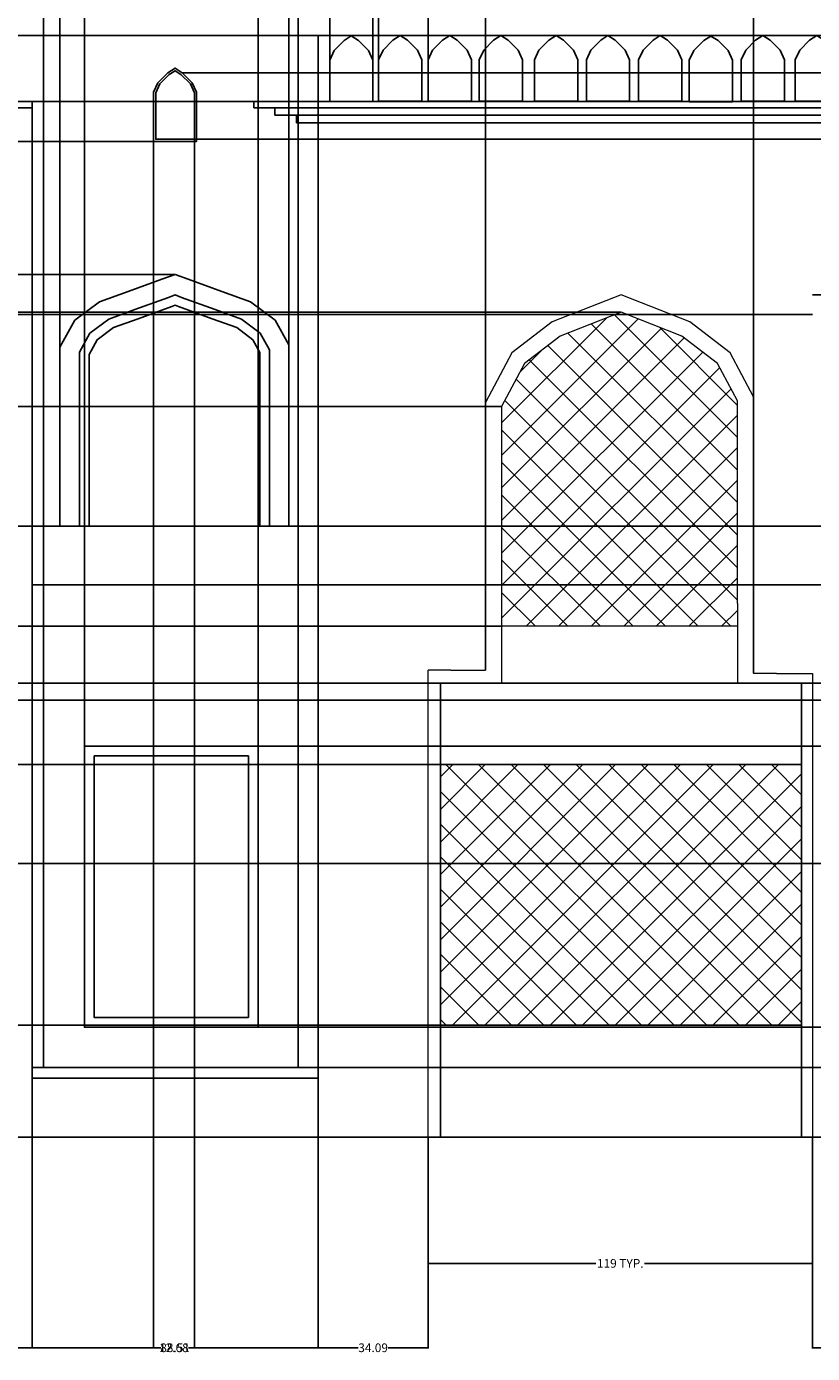
# Model space of a CAD drawing. Units: inches. Extents: x 2 to 1442, y 20 to 729.
# Tile 3 of 8: x 343 to 586, y 20 to 431. Entities that reach past the tile are written whole.
import ezdxf

# ---------------------------------------------------------------- set-up
doc = ezdxf.new("R2010")
doc.units = ezdxf.units.IN
doc.header["$MEASUREMENT"] = 0
for name, color, linetype, lineweight in [('A-ANNO-DIMS', 2, 'Continuous', 18), ('A-ELEV', 7, 'Continuous', 25), ('A-GLAZ', 4, 'Continuous', 18), ('A-GLAZ-PATT', 9, 'Continuous', 13)]:
    doc.layers.add(name, color=color, linetype=linetype, lineweight=lineweight)
doc.styles.get("Standard").update_dxf_attribs({"font": 'arial.ttf'})
doc.dimstyles.get("Standard").update_dxf_attribs({"dimtxt": 2.6875, "dimasz": 0.18, "dimexe": 0.18, "dimexo": 0.0625, "dimgap": 0.09, "dimtad": 0, "dimtih": 1, "dimtoh": 1, "dimdec": 4, "dimzin": 0, "dimdsep": 46, "dimlunit": 4, "dimtxsty": 'Standard', "dimcen": 0.09, "dimadec": 0, "dimazin": 0, "dimtfac": 1, "dimtdec": 4, "dimtofl": 0, "dimtmove": 0, "dimatfit": 3, "dimfxl": 1, "dimtolj": 1, "dimtzin": 0, "dimarcsym": 0})

# ---------------------------------------------------------------- blocks, each defined once
blk = doc.blocks.new('WIN-JALI-PANEL')
for p, q in [((17.71, 144.52), (17.71, 165.38)), ((22.71, 165.38), (22.71, 158.15)), ((95.66, 165.25), (95.66, 158.15)), ((100.66, 165.25), (100.66, 143.52)), ((95.66, 158.15), (22.71, 158.15)), ((22.71, 158.15), (22.71, 140.52)), ((95.66, 158.15), (95.66, 140.52)), ((0, 0), (0, 144.52)), ((7.01, 144.52), (0, 144.52)), ((7.01, 144.52), (17.71, 144.52)), ((107.81, 143.52), (100.66, 143.52)), ((107.81, 143.52), (118.87, 143.52)), ((118.87, 143.52), (118.87, 100.88)), ((118.87, 100.88), (118.87, 0))]:
    blk.add_line(p, q)
for points in [[(100.66, 165.25), (100.66, 224.45), (100.65, 229.2), (93.44, 242.86), (80.93, 252.42), (59.66, 260.79), (38.39, 252.42), (25.88, 242.86), (17.71, 227.39), (17.71, 165.38)], [(95.66, 165.25), (95.66, 224.45), (95.66, 227.96), (89.53, 239.55), (78.45, 248.02), (59.66, 255.41), (40.87, 248.02), (29.79, 239.55), (22.71, 226.15), (22.71, 165.38)]]:
    blk.add_lwpolyline(points)
blk = doc.blocks.new('*D9')
at = {"layer": 'A-ANNO-DIMS', "color": 0, "lineweight": -2, "transparency": 16777216}
for p, q in [((585.99, 348.06), (625.22, 348.06)), ((625.04, 347.88), (625.04, 219.14)), ((625.04, 87.45), (625.04, 216.18)), ((585.99, 87.27), (625.22, 87.27))]:
    blk.add_line(p, q, dxfattribs=at)
at = {"layer": 'A-ANNO-DIMS', "color": 0, "transparency": 16777216}
for points in [[(625.01, 347.88), (625.07, 347.88), (625.04, 348.06)], [(625.01, 87.45), (625.07, 87.45), (625.04, 87.27)]]:
    blk.add_solid(points, dxfattribs=at)
at = {"layer": 'Defpoints', "color": 0, "transparency": 16777216}
for p in [(585.93, 348.06), (625.04, 348.06), (585.93, 87.27)]:
    blk.add_point(p, dxfattribs=at)
at = {"layer": 'A-ANNO-DIMS', "color": 0, "transparency": 16777216, "insert": (625.04, 217.66), "char_height": 2.6875, "attachment_point": 5}
blk.add_mtext('\\A1;JALI SCREEN 261 TYP.', dxfattribs=at)
blk = doc.blocks.new('*D10')
at = {"layer": 'A-ANNO-DIMS', "color": 0, "lineweight": -2, "transparency": 16777216}
for p, q in [((467.06, 87.21), (467.06, 47.97)), ((585.93, 87.21), (585.93, 47.97)), ((467.24, 48.15), (518.94, 48.15)), ((585.75, 48.15), (534.04, 48.15))]:
    blk.add_line(p, q, dxfattribs=at)
at = {"layer": 'A-ANNO-DIMS', "color": 0, "transparency": 16777216}
for points in [[(467.24, 48.18), (467.24, 48.12), (467.06, 48.15)], [(585.75, 48.18), (585.75, 48.12), (585.93, 48.15)]]:
    blk.add_solid(points, dxfattribs=at)
at = {"layer": 'Defpoints', "color": 0, "transparency": 16777216}
for p in [(467.06, 87.27), (585.93, 87.27), (585.93, 48.15)]:
    blk.add_point(p, dxfattribs=at)
at = {"layer": 'A-ANNO-DIMS', "color": 0, "transparency": 16777216, "insert": (526.49, 48.15), "char_height": 2.6875, "attachment_point": 5}
blk.add_mtext('\\A1;119 TYP.', dxfattribs=at)
blk = doc.blocks.new('*D18')
at = {"layer": 'A-ANNO-DIMS', "color": 0, "lineweight": -2, "transparency": 16777216}
for p, q in [((318.25, 87.21), (318.25, 21.84)), ((344.45, 87.21), (344.45, 21.84)), ((318.43, 22.02), (325.66, 22.02)), ((344.27, 22.02), (337.04, 22.02))]:
    blk.add_line(p, q, dxfattribs=at)
at = {"layer": 'A-ANNO-DIMS', "color": 0, "transparency": 16777216}
for points in [[(318.43, 22.05), (318.43, 21.99), (318.25, 22.02)], [(344.27, 22.05), (344.27, 21.99), (344.45, 22.02)]]:
    blk.add_solid(points, dxfattribs=at)
at = {"layer": 'Defpoints', "color": 0, "transparency": 16777216}
for p in [(318.25, 87.27), (344.45, 87.27), (344.45, 22.02)]:
    blk.add_point(p, dxfattribs=at)
at = {"layer": 'A-ANNO-DIMS', "color": 0, "transparency": 16777216, "insert": (331.35, 22.02), "char_height": 2.688, "attachment_point": 5}
blk.add_mtext('\\A1;26.204', dxfattribs=at)
blk = doc.blocks.new('*D19')
at = {"layer": 'A-ANNO-DIMS', "color": 0, "lineweight": -2, "transparency": 16777216}
for p, q in [((344.45, 87.21), (344.45, 21.84)), ((432.97, 87.21), (432.97, 21.84)), ((344.63, 22.02), (384.34, 22.02)), ((432.79, 22.02), (393.08, 22.02))]:
    blk.add_line(p, q, dxfattribs=at)
at = {"layer": 'A-ANNO-DIMS', "color": 0, "transparency": 16777216}
for points in [[(344.63, 22.05), (344.63, 21.99), (344.45, 22.02)], [(432.79, 22.05), (432.79, 21.99), (432.97, 22.02)]]:
    blk.add_solid(points, dxfattribs=at)
at = {"layer": 'Defpoints', "color": 0, "transparency": 16777216}
for p in [(344.45, 87.27), (432.97, 87.27), (432.97, 22.02)]:
    blk.add_point(p, dxfattribs=at)
at = {"layer": 'A-ANNO-DIMS', "color": 0, "transparency": 16777216, "insert": (388.71, 22.02), "char_height": 2.688, "attachment_point": 5}
blk.add_mtext('\\A1;88.51', dxfattribs=at)
blk = doc.blocks.new('*D20')
at = {"layer": 'A-ANNO-DIMS', "color": 0, "lineweight": -2, "transparency": 16777216}
for p, q in [((432.97, 87.21), (432.97, 21.84)), ((467.06, 87.21), (467.06, 21.84)), ((433.15, 22.02), (445.39, 22.02)), ((466.88, 22.02), (454.64, 22.02))]:
    blk.add_line(p, q, dxfattribs=at)
at = {"layer": 'A-ANNO-DIMS', "color": 0, "transparency": 16777216}
for points in [[(433.15, 22.05), (433.15, 21.99), (432.97, 22.02)], [(466.88, 22.05), (466.88, 21.99), (467.06, 22.02)]]:
    blk.add_solid(points, dxfattribs=at)
at = {"layer": 'Defpoints', "color": 0, "transparency": 16777216}
for p in [(432.97, 87.27), (467.06, 87.27), (467.06, 22.02)]:
    blk.add_point(p, dxfattribs=at)
at = {"layer": 'A-ANNO-DIMS', "color": 0, "transparency": 16777216, "insert": (450.01, 22.02), "char_height": 2.688, "attachment_point": 5}
blk.add_mtext('\\A1;34.09', dxfattribs=at)
blk = doc.blocks.new('*D21')
at = {"layer": 'A-ANNO-DIMS', "color": 0, "lineweight": -2, "transparency": 16777216}
for p, q in [((585.93, 87.21), (585.93, 21.84)), ((656, 87.21), (656, 21.84)), ((586.11, 22.02), (616.35, 22.02)), ((655.82, 22.02), (625.58, 22.02))]:
    blk.add_line(p, q, dxfattribs=at)
at = {"layer": 'A-ANNO-DIMS', "color": 0, "transparency": 16777216}
for points in [[(586.11, 22.05), (586.11, 21.99), (585.93, 22.02)], [(655.82, 22.05), (655.82, 21.99), (656, 22.02)]]:
    blk.add_solid(points, dxfattribs=at)
at = {"layer": 'Defpoints', "color": 0, "transparency": 16777216}
for p in [(585.93, 87.27), (656, 87.27), (656, 22.02)]:
    blk.add_point(p, dxfattribs=at)
at = {"layer": 'A-ANNO-DIMS', "color": 0, "transparency": 16777216, "insert": (620.96, 22.02), "char_height": 2.688, "attachment_point": 5}
blk.add_mtext('\\A1;70.07', dxfattribs=at)
blk = doc.blocks.new('*D49')
at = {"layer": 'A-ANNO-DIMS', "color": 0, "lineweight": -2, "transparency": 16777216}
for p, q in [((353.09, 276.51), (353.09, 726.93)), ((353.27, 726.75), (383.9, 726.75)), ((423.76, 726.75), (393.14, 726.75)), ((423.94, 276.51), (423.94, 726.93))]:
    blk.add_line(p, q, dxfattribs=at)
at = {"layer": 'A-ANNO-DIMS', "color": 0, "transparency": 16777216}
for points in [[(353.27, 726.78), (353.27, 726.72), (353.09, 726.75)], [(423.76, 726.78), (423.76, 726.72), (423.94, 726.75)]]:
    blk.add_solid(points, dxfattribs=at)
at = {"layer": 'Defpoints', "color": 0, "transparency": 16777216}
for p in [(423.94, 726.75), (353.09, 276.44), (423.94, 276.44)]:
    blk.add_point(p, dxfattribs=at)
at = {"layer": 'A-ANNO-DIMS', "color": 0, "transparency": 16777216, "insert": (388.52, 726.75), "char_height": 2.688, "attachment_point": 5}
blk.add_mtext('\\A1;70.85', dxfattribs=at)
blk = doc.blocks.new('*D50')
at = {"layer": 'A-ANNO-DIMS', "color": 0, "lineweight": -2, "transparency": 16777216}
for p, q in [((433.03, 108.8), (1436.55, 108.8)), ((1436.37, 108.62), (1436.37, 99.5)), ((1436.37, 87.45), (1436.37, 96.57)), ((433.03, 87.27), (1436.55, 87.27))]:
    blk.add_line(p, q, dxfattribs=at)
at = {"layer": 'A-ANNO-DIMS', "color": 0, "transparency": 16777216}
for points in [[(1436.34, 108.62), (1436.4, 108.62), (1436.37, 108.8)], [(1436.34, 87.45), (1436.4, 87.45), (1436.37, 87.27)]]:
    blk.add_solid(points, dxfattribs=at)
at = {"layer": 'Defpoints', "color": 0, "transparency": 16777216}
for p in [(432.97, 108.8), (1436.37, 108.8), (432.97, 87.27)]:
    blk.add_point(p, dxfattribs=at)
at = {"layer": 'A-ANNO-DIMS', "color": 0, "transparency": 16777216, "insert": (1436.37, 98.04), "char_height": 2.688, "attachment_point": 5}
blk.add_mtext('\\A1;21.53', dxfattribs=at)
blk = doc.blocks.new('*D51')
at = {"layer": 'A-ANNO-DIMS', "color": 0, "lineweight": -2, "transparency": 16777216}
for p, q in [((426.83, 227.79), (1436.55, 227.79)), ((1436.37, 227.61), (1436.37, 169.76)), ((1436.37, 108.98), (1436.37, 166.83)), ((433.03, 108.8), (1436.55, 108.8))]:
    blk.add_line(p, q, dxfattribs=at)
at = {"layer": 'A-ANNO-DIMS', "color": 0, "transparency": 16777216}
for points in [[(1436.34, 227.61), (1436.4, 227.61), (1436.37, 227.79)], [(1436.34, 108.98), (1436.4, 108.98), (1436.37, 108.8)]]:
    blk.add_solid(points, dxfattribs=at)
at = {"layer": 'Defpoints', "color": 0, "transparency": 16777216}
for p in [(426.77, 227.79), (1436.37, 227.79), (432.97, 108.8)]:
    blk.add_point(p, dxfattribs=at)
at = {"layer": 'A-ANNO-DIMS', "color": 0, "transparency": 16777216, "insert": (1436.37, 168.3), "char_height": 2.688, "attachment_point": 5}
blk.add_mtext('\\A1;118.99', dxfattribs=at)
blk = doc.blocks.new('*D52')
at = {"layer": 'A-ANNO-DIMS', "color": 0, "lineweight": -2, "transparency": 16777216}
for p, q in [((433.03, 258.25), (1436.55, 258.25)), ((1436.37, 258.07), (1436.37, 244.49)), ((1436.37, 227.97), (1436.37, 241.56)), ((426.83, 227.79), (1436.55, 227.79))]:
    blk.add_line(p, q, dxfattribs=at)
at = {"layer": 'A-ANNO-DIMS', "color": 0, "transparency": 16777216}
for points in [[(1436.34, 258.07), (1436.4, 258.07), (1436.37, 258.25)], [(1436.34, 227.97), (1436.4, 227.97), (1436.37, 227.79)]]:
    blk.add_solid(points, dxfattribs=at)
at = {"layer": 'Defpoints', "color": 0, "transparency": 16777216}
for p in [(432.97, 258.25), (1436.37, 258.25), (426.77, 227.79)]:
    blk.add_point(p, dxfattribs=at)
at = {"layer": 'A-ANNO-DIMS', "color": 0, "transparency": 16777216, "insert": (1436.37, 243.02), "char_height": 2.688, "attachment_point": 5}
blk.add_mtext('\\A1;30.464', dxfattribs=at)
blk = doc.blocks.new('*D53')
at = {"layer": 'A-ANNO-DIMS', "color": 0, "lineweight": -2, "transparency": 16777216}
for p, q in [((433.03, 276.44), (1436.55, 276.44)), ((1436.37, 276.26), (1436.37, 268.81)), ((1436.37, 258.43), (1436.37, 265.89)), ((433.03, 258.25), (1436.55, 258.25))]:
    blk.add_line(p, q, dxfattribs=at)
at = {"layer": 'A-ANNO-DIMS', "color": 0, "transparency": 16777216}
for points in [[(1436.34, 276.26), (1436.4, 276.26), (1436.37, 276.44)], [(1436.34, 258.43), (1436.4, 258.43), (1436.37, 258.25)]]:
    blk.add_solid(points, dxfattribs=at)
at = {"layer": 'Defpoints', "color": 0, "transparency": 16777216}
for p in [(432.97, 276.44), (1436.37, 276.44), (432.97, 258.25)]:
    blk.add_point(p, dxfattribs=at)
at = {"layer": 'A-ANNO-DIMS', "color": 0, "transparency": 16777216, "insert": (1436.37, 267.35), "char_height": 2.688, "attachment_point": 5}
blk.add_mtext('\\A1;18.19', dxfattribs=at)
blk = doc.blocks.new('*D54')
at = {"layer": 'A-ANNO-DIMS', "color": 0, "lineweight": -2, "transparency": 16777216}
for p, q in [((388.65, 354.39), (7.1, 354.39)), ((7.28, 354.21), (7.28, 316.88)), ((7.28, 276.62), (7.28, 313.95)), ((353.03, 276.44), (7.1, 276.44))]:
    blk.add_line(p, q, dxfattribs=at)
at = {"layer": 'A-ANNO-DIMS', "color": 0, "transparency": 16777216}
for points in [[(7.25, 354.21), (7.31, 354.21), (7.28, 354.39)], [(7.25, 276.62), (7.31, 276.62), (7.28, 276.44)]]:
    blk.add_solid(points, dxfattribs=at)
at = {"layer": 'Defpoints', "color": 0, "transparency": 16777216}
for p in [(7.28, 354.39), (388.71, 354.39), (353.09, 276.44)]:
    blk.add_point(p, dxfattribs=at)
at = {"layer": 'A-ANNO-DIMS', "color": 0, "transparency": 16777216, "insert": (7.28, 315.41), "char_height": 2.688, "attachment_point": 5}
blk.add_mtext('\\A1;77.94', dxfattribs=at)
blk = doc.blocks.new('*D55')
at = {"layer": 'A-ANNO-DIMS', "color": 0, "lineweight": -2, "transparency": 16777216}
for p, q in [((391.01, 416.82), (1436.55, 416.82)), ((1436.37, 416.64), (1436.37, 407.98)), ((1436.37, 396.4), (1436.37, 405.06)), ((394.77, 396.22), (1436.55, 396.22))]:
    blk.add_line(p, q, dxfattribs=at)
at = {"layer": 'A-ANNO-DIMS', "color": 0, "transparency": 16777216}
for points in [[(1436.34, 416.64), (1436.4, 416.64), (1436.37, 416.82)], [(1436.34, 396.4), (1436.4, 396.4), (1436.37, 396.22)]]:
    blk.add_solid(points, dxfattribs=at)
at = {"layer": 'Defpoints', "color": 0, "transparency": 16777216}
for p in [(390.95, 416.82), (1436.37, 416.82), (394.7, 396.22)]:
    blk.add_point(p, dxfattribs=at)
at = {"layer": 'A-ANNO-DIMS', "color": 0, "transparency": 16777216, "insert": (1436.37, 406.52), "char_height": 2.688, "attachment_point": 5}
blk.add_mtext('\\A1;20.605', dxfattribs=at)
blk = doc.blocks.new('*D56')
at = {"layer": 'A-ANNO-DIMS', "color": 0, "lineweight": -2, "transparency": 16777216}
for p, q in [((382.02, 395.46), (382.02, 21.84)), ((394.7, 396.15), (394.7, 21.84)), ((382.2, 22.02), (383.86, 22.02)), ((394.52, 22.02), (392.86, 22.02))]:
    blk.add_line(p, q, dxfattribs=at)
at = {"layer": 'A-ANNO-DIMS', "color": 0, "transparency": 16777216}
for points in [[(382.2, 22.05), (382.2, 21.99), (382.02, 22.02)], [(394.52, 22.05), (394.52, 21.99), (394.7, 22.02)]]:
    blk.add_solid(points, dxfattribs=at)
at = {"layer": 'Defpoints', "color": 0, "transparency": 16777216}
for p in [(382.02, 395.53), (394.7, 396.22), (394.7, 22.02)]:
    blk.add_point(p, dxfattribs=at)
at = {"layer": 'A-ANNO-DIMS', "color": 0, "transparency": 16777216, "insert": (388.36, 22.02), "char_height": 2.688, "attachment_point": 5}
blk.add_mtext('\\A1;12.68', dxfattribs=at)
blk = doc.blocks.new('*D57')
at = {"layer": 'A-ANNO-DIMS', "color": 0, "lineweight": -2, "transparency": 16777216}
for p, q in [((381.96, 395.53), (7.1, 395.53)), ((7.28, 395.35), (7.28, 376.4)), ((7.28, 354.57), (7.28, 373.52)), ((388.65, 354.39), (7.1, 354.39))]:
    blk.add_line(p, q, dxfattribs=at)
at = {"layer": 'A-ANNO-DIMS', "color": 0, "transparency": 16777216}
for points in [[(7.25, 395.35), (7.31, 395.35), (7.28, 395.53)], [(7.25, 354.57), (7.31, 354.57), (7.28, 354.39)]]:
    blk.add_solid(points, dxfattribs=at)
at = {"layer": 'Defpoints', "color": 0, "transparency": 16777216}
for p in [(382.02, 395.53), (7.28, 354.39), (388.71, 354.39)]:
    blk.add_point(p, dxfattribs=at)
at = {"layer": 'A-ANNO-DIMS', "color": 0, "transparency": 16777216, "insert": (7.28, 374.96), "char_height": 2.688, "attachment_point": 5}
blk.add_mtext('\\A1;41.14', dxfattribs=at)
blk = doc.blocks.new('*D58')
at = {"layer": 'A-ANNO-DIMS', "color": 0, "lineweight": -2, "transparency": 16777216}
for p, q in [((347.98, 227.85), (347.98, 726.93)), ((348.16, 726.75), (382.76, 726.75)), ((426.59, 726.75), (391.99, 726.75)), ((426.77, 227.85), (426.77, 726.93))]:
    blk.add_line(p, q, dxfattribs=at)
at = {"layer": 'A-ANNO-DIMS', "color": 0, "transparency": 16777216}
for points in [[(348.16, 726.78), (348.16, 726.72), (347.98, 726.75)], [(426.59, 726.78), (426.59, 726.72), (426.77, 726.75)]]:
    blk.add_solid(points, dxfattribs=at)
at = {"layer": 'Defpoints', "color": 0, "transparency": 16777216}
for p in [(426.77, 726.75), (347.98, 227.79), (426.77, 227.79)]:
    blk.add_point(p, dxfattribs=at)
at = {"layer": 'A-ANNO-DIMS', "color": 0, "transparency": 16777216, "insert": (387.38, 726.75), "char_height": 2.688, "attachment_point": 5}
blk.add_mtext('\\A1;78.79', dxfattribs=at)
blk = doc.blocks.new('*D59')
at = {"layer": 'A-ANNO-DIMS', "color": 0, "lineweight": -2, "transparency": 16777216}
for p, q in [((360.68, 208.33), (360.68, 726.93)), ((360.86, 726.75), (382.91, 726.75)), ((414.24, 726.75), (392.18, 726.75)), ((414.42, 208.33), (414.42, 726.93))]:
    blk.add_line(p, q, dxfattribs=at)
at = {"layer": 'A-ANNO-DIMS', "color": 0, "transparency": 16777216}
for points in [[(360.86, 726.78), (360.86, 726.72), (360.68, 726.75)], [(414.24, 726.78), (414.24, 726.72), (414.42, 726.75)]]:
    blk.add_solid(points, dxfattribs=at)
at = {"layer": 'Defpoints', "color": 0, "transparency": 16777216}
for p in [(414.42, 726.75), (360.68, 208.27), (414.42, 208.27)]:
    blk.add_point(p, dxfattribs=at)
at = {"layer": 'A-ANNO-DIMS', "color": 0, "transparency": 16777216, "insert": (387.55, 726.75), "char_height": 2.688, "attachment_point": 5}
blk.add_mtext('\\A1;53.75', dxfattribs=at)
blk = doc.blocks.new('*D60')
at = {"layer": 'A-ANNO-DIMS', "color": 0, "lineweight": -2, "transparency": 16777216}
for p, q in [((414.48, 208.27), (1436.55, 208.27)), ((1436.37, 208.09), (1436.37, 166.24)), ((1436.37, 121.46), (1436.37, 163.32)), ((414.48, 121.28), (1436.55, 121.28))]:
    blk.add_line(p, q, dxfattribs=at)
at = {"layer": 'A-ANNO-DIMS', "color": 0, "transparency": 16777216}
for points in [[(1436.34, 208.09), (1436.4, 208.09), (1436.37, 208.27)], [(1436.34, 121.46), (1436.4, 121.46), (1436.37, 121.28)]]:
    blk.add_solid(points, dxfattribs=at)
at = {"layer": 'Defpoints', "color": 0, "transparency": 16777216}
for p in [(414.42, 208.27), (1436.37, 208.27), (414.42, 121.28)]:
    blk.add_point(p, dxfattribs=at)
at = {"layer": 'A-ANNO-DIMS', "color": 0, "transparency": 16777216, "insert": (1436.37, 164.78), "char_height": 2.688, "attachment_point": 5}
blk.add_mtext('\\A1;86.99', dxfattribs=at)
blk = doc.blocks.new('*D61')
at = {"layer": 'A-ANNO-DIMS', "color": 0, "lineweight": -2, "transparency": 16777216}
for p, q in [((432.9, 428.31), (7.1, 428.31)), ((7.28, 428.13), (7.28, 419.56)), ((7.28, 408.07), (7.28, 416.64)), ((432.9, 407.89), (7.1, 407.89))]:
    blk.add_line(p, q, dxfattribs=at)
at = {"layer": 'A-ANNO-DIMS', "color": 0, "transparency": 16777216}
for points in [[(7.25, 428.13), (7.31, 428.13), (7.28, 428.31)], [(7.25, 408.07), (7.31, 408.07), (7.28, 407.89)]]:
    blk.add_solid(points, dxfattribs=at)
at = {"layer": 'Defpoints', "color": 0, "transparency": 16777216}
for p in [(7.28, 428.31), (432.97, 428.31), (432.97, 407.89)]:
    blk.add_point(p, dxfattribs=at)
at = {"layer": 'A-ANNO-DIMS', "color": 0, "transparency": 16777216, "insert": (7.28, 418.1), "char_height": 2.688, "attachment_point": 5}
blk.add_mtext('\\A1;20.426', dxfattribs=at)
blk = doc.blocks.new('*D62')
at = {"layer": 'A-ANNO-DIMS', "color": 0, "lineweight": -2, "transparency": 16777216}
for p, q in [((436.57, 420.81), (436.57, 726.93)), ((436.75, 726.75), (438.76, 726.75)), ((449.76, 726.75), (447.75, 726.75)), ((449.94, 420.81), (449.94, 726.93))]:
    blk.add_line(p, q, dxfattribs=at)
at = {"layer": 'A-ANNO-DIMS', "color": 0, "transparency": 16777216}
for points in [[(436.75, 726.78), (436.75, 726.72), (436.57, 726.75)], [(449.76, 726.78), (449.76, 726.72), (449.94, 726.75)]]:
    blk.add_solid(points, dxfattribs=at)
at = {"layer": 'Defpoints', "color": 0, "transparency": 16777216}
for p in [(449.94, 726.75), (436.57, 420.75), (449.94, 420.75)]:
    blk.add_point(p, dxfattribs=at)
at = {"layer": 'A-ANNO-DIMS', "color": 0, "transparency": 16777216, "insert": (443.26, 726.75), "char_height": 2.688, "attachment_point": 5}
blk.add_mtext('\\A1;13.37', dxfattribs=at)
blk = doc.blocks.new('*D63')
at = {"layer": 'A-ANNO-DIMS', "color": 0, "lineweight": -2, "transparency": 16777216}
for p, q in [((451.71, 420.89), (451.71, 726.93)), ((451.89, 726.75), (454.89, 726.75)), ((466.88, 726.75), (463.88, 726.75)), ((467.06, 420.89), (467.06, 726.93))]:
    blk.add_line(p, q, dxfattribs=at)
at = {"layer": 'A-ANNO-DIMS', "color": 0, "transparency": 16777216}
for points in [[(451.89, 726.78), (451.89, 726.72), (451.71, 726.75)], [(466.88, 726.78), (466.88, 726.72), (467.06, 726.75)]]:
    blk.add_solid(points, dxfattribs=at)
at = {"layer": 'Defpoints', "color": 0, "transparency": 16777216}
for p in [(467.06, 726.75), (451.71, 420.83), (467.06, 420.83)]:
    blk.add_point(p, dxfattribs=at)
at = {"layer": 'A-ANNO-DIMS', "color": 0, "transparency": 16777216, "insert": (459.39, 726.75), "char_height": 2.688, "attachment_point": 5}
blk.add_mtext('\\A1;15.34', dxfattribs=at)
blk = doc.blocks.new('*D72')
at = {"layer": 'A-ANNO-DIMS', "color": 0, "lineweight": -2, "transparency": 16777216}
for p, q in [((585.94, 341.99), (7.1, 341.99)), ((7.28, 341.81), (7.28, 216.09)), ((7.28, 87.45), (7.28, 213.17)), ((592.44, 87.27), (7.1, 87.27))]:
    blk.add_line(p, q, dxfattribs=at)
at = {"layer": 'A-ANNO-DIMS', "color": 0, "transparency": 16777216}
for points in [[(7.25, 341.81), (7.31, 341.81), (7.28, 341.99)], [(7.25, 87.45), (7.31, 87.45), (7.28, 87.27)]]:
    blk.add_solid(points, dxfattribs=at)
at = {"layer": 'Defpoints', "color": 0, "transparency": 16777216}
for p in [(7.28, 341.99), (586, 341.99), (592.5, 87.27)]:
    blk.add_point(p, dxfattribs=at)
at = {"layer": 'A-ANNO-DIMS', "color": 0, "transparency": 16777216, "insert": (7.28, 214.63), "char_height": 2.688, "attachment_point": 5}
blk.add_mtext('\\A1;254.7', dxfattribs=at)
blk = doc.blocks.new('*D74')
at = {"layer": 'A-ANNO-DIMS', "color": 0, "lineweight": -2, "transparency": 16777216}
for p, q in [((655.94, 172), (7.1, 172)), ((7.28, 171.82), (7.28, 131.1)), ((7.28, 87.45), (7.28, 128.17)), ((655.94, 87.27), (7.1, 87.27))]:
    blk.add_line(p, q, dxfattribs=at)
at = {"layer": 'A-ANNO-DIMS', "color": 0, "transparency": 16777216}
for points in [[(7.25, 171.82), (7.31, 171.82), (7.28, 172)], [(7.25, 87.45), (7.31, 87.45), (7.28, 87.27)]]:
    blk.add_solid(points, dxfattribs=at)
at = {"layer": 'Defpoints', "color": 0, "transparency": 16777216}
for p in [(656, 172), (7.28, 87.27), (656, 87.27)]:
    blk.add_point(p, dxfattribs=at)
at = {"layer": 'A-ANNO-DIMS', "color": 0, "transparency": 16777216, "insert": (7.28, 129.64), "char_height": 2.688, "attachment_point": 5}
blk.add_mtext('\\A1;84.73', dxfattribs=at)
blk = doc.blocks.new('*D75')
at = {"layer": 'A-ANNO-DIMS', "color": 0, "lineweight": -2, "transparency": 16777216}
for p, q in [((721.76, 222.5), (7.1, 222.5)), ((7.28, 222.32), (7.28, 198.71)), ((7.28, 172.18), (7.28, 195.79)), ((655.94, 172), (7.1, 172))]:
    blk.add_line(p, q, dxfattribs=at)
at = {"layer": 'A-ANNO-DIMS', "color": 0, "transparency": 16777216}
for points in [[(7.25, 222.32), (7.31, 222.32), (7.28, 222.5)], [(7.25, 172.18), (7.31, 172.18), (7.28, 172)]]:
    blk.add_solid(points, dxfattribs=at)
at = {"layer": 'Defpoints', "color": 0, "transparency": 16777216}
for p in [(7.28, 222.5), (721.83, 222.5), (656, 172)]:
    blk.add_point(p, dxfattribs=at)
at = {"layer": 'A-ANNO-DIMS', "color": 0, "transparency": 16777216, "insert": (7.28, 197.25), "char_height": 2.688, "attachment_point": 5}
blk.add_mtext('\\A1;50.5', dxfattribs=at)
blk = doc.blocks.new('*D76')
at = {"layer": 'A-ANNO-DIMS', "color": 0, "lineweight": -2, "transparency": 16777216}
for p, q in [((470.75, 121.87), (7.1, 121.87)), ((7.28, 121.69), (7.28, 106.03)), ((7.28, 87.45), (7.28, 103.11)), ((470.75, 87.27), (7.1, 87.27))]:
    blk.add_line(p, q, dxfattribs=at)
at = {"layer": 'A-ANNO-DIMS', "color": 0, "transparency": 16777216}
for points in [[(7.25, 121.69), (7.31, 121.69), (7.28, 121.87)], [(7.25, 87.45), (7.31, 87.45), (7.28, 87.27)]]:
    blk.add_solid(points, dxfattribs=at)
at = {"layer": 'Defpoints', "color": 0, "transparency": 16777216}
for p in [(470.81, 121.87), (7.28, 87.27), (470.81, 87.27)]:
    blk.add_point(p, dxfattribs=at)
at = {"layer": 'A-ANNO-DIMS', "color": 0, "transparency": 16777216, "insert": (7.28, 104.57), "char_height": 2.688, "attachment_point": 5}
blk.add_mtext('\\A1;34.6', dxfattribs=at)
blk = doc.blocks.new('*D77')
at = {"layer": 'A-ANNO-DIMS', "color": 0, "lineweight": -2, "transparency": 16777216}
for p, q in [((470.75, 202.58), (7.1, 202.58)), ((7.28, 202.4), (7.28, 163.69)), ((7.28, 122.05), (7.28, 160.77)), ((470.75, 121.87), (7.1, 121.87))]:
    blk.add_line(p, q, dxfattribs=at)
at = {"layer": 'A-ANNO-DIMS', "color": 0, "transparency": 16777216}
for points in [[(7.25, 202.4), (7.31, 202.4), (7.28, 202.58)], [(7.25, 122.05), (7.31, 122.05), (7.28, 121.87)]]:
    blk.add_solid(points, dxfattribs=at)
at = {"layer": 'Defpoints', "color": 0, "transparency": 16777216}
for p in [(7.28, 202.58), (470.81, 202.58), (470.81, 121.87)]:
    blk.add_point(p, dxfattribs=at)
at = {"layer": 'A-ANNO-DIMS', "color": 0, "transparency": 16777216, "insert": (7.28, 162.23), "char_height": 2.688, "attachment_point": 5}
blk.add_mtext('\\A1;80.71', dxfattribs=at)
blk = doc.blocks.new('*D78')
at = {"layer": 'A-ANNO-DIMS', "color": 0, "lineweight": -2, "transparency": 16777216}
for p, q in [((470.75, 227.79), (7.1, 227.79)), ((7.28, 227.61), (7.28, 216.65)), ((7.28, 202.76), (7.28, 213.72)), ((470.75, 202.58), (7.1, 202.58))]:
    blk.add_line(p, q, dxfattribs=at)
at = {"layer": 'A-ANNO-DIMS', "color": 0, "transparency": 16777216}
for points in [[(7.25, 227.61), (7.31, 227.61), (7.28, 227.79)], [(7.25, 202.76), (7.31, 202.76), (7.28, 202.58)]]:
    blk.add_solid(points, dxfattribs=at)
at = {"layer": 'Defpoints', "color": 0, "transparency": 16777216}
for p in [(7.28, 227.79), (470.81, 227.79), (470.81, 202.58)]:
    blk.add_point(p, dxfattribs=at)
at = {"layer": 'A-ANNO-DIMS', "color": 0, "transparency": 16777216, "insert": (7.28, 215.19), "char_height": 2.688, "attachment_point": 5}
blk.add_mtext('\\A1;25.206', dxfattribs=at)
blk = doc.blocks.new('*D79')
at = {"layer": 'A-ANNO-DIMS', "color": 0, "lineweight": -2, "transparency": 16777216}
for p, q in [((489.71, 313.43), (7.1, 313.43)), ((7.28, 313.25), (7.28, 280.88)), ((7.28, 245.6), (7.28, 277.96)), ((489.71, 245.42), (7.1, 245.42))]:
    blk.add_line(p, q, dxfattribs=at)
at = {"layer": 'A-ANNO-DIMS', "color": 0, "transparency": 16777216}
for points in [[(7.25, 313.25), (7.31, 313.25), (7.28, 313.43)], [(7.25, 245.6), (7.31, 245.6), (7.28, 245.42)]]:
    blk.add_solid(points, dxfattribs=at)
at = {"layer": 'Defpoints', "color": 0, "transparency": 16777216}
for p in [(7.28, 313.43), (489.77, 313.43), (489.77, 245.42)]:
    blk.add_point(p, dxfattribs=at)
at = {"layer": 'A-ANNO-DIMS', "color": 0, "transparency": 16777216, "insert": (7.28, 279.42), "char_height": 2.688, "attachment_point": 5}
blk.add_mtext('\\A1;68', dxfattribs=at)
blk = doc.blocks.new('*D80')
at = {"layer": 'A-ANNO-DIMS', "color": 0, "lineweight": -2, "transparency": 16777216}
for p, q in [((526.66, 342.68), (7.1, 342.68)), ((7.28, 342.5), (7.28, 329.52)), ((7.28, 313.61), (7.28, 326.59)), ((489.71, 313.43), (7.1, 313.43))]:
    blk.add_line(p, q, dxfattribs=at)
at = {"layer": 'A-ANNO-DIMS', "color": 0, "transparency": 16777216}
for points in [[(7.25, 342.5), (7.31, 342.5), (7.28, 342.68)], [(7.25, 313.61), (7.31, 313.61), (7.28, 313.43)]]:
    blk.add_solid(points, dxfattribs=at)
at = {"layer": 'Defpoints', "color": 0, "transparency": 16777216}
for p in [(7.28, 342.68), (526.72, 342.68), (489.77, 313.43)]:
    blk.add_point(p, dxfattribs=at)
at = {"layer": 'A-ANNO-DIMS', "color": 0, "transparency": 16777216, "insert": (7.28, 328.05), "char_height": 2.688, "attachment_point": 5}
blk.add_mtext('\\A1;29.26', dxfattribs=at)
blk = doc.blocks.new('*D81')
at = {"layer": 'A-ANNO-DIMS', "color": 0, "lineweight": -2, "transparency": 16777216}
for p, q in [((484.77, 231.85), (484.77, 726.93)), ((484.95, 726.75), (521.61, 726.75)), ((567.54, 726.75), (530.88, 726.75)), ((567.72, 230.85), (567.72, 726.93))]:
    blk.add_line(p, q, dxfattribs=at)
at = {"layer": 'A-ANNO-DIMS', "color": 0, "transparency": 16777216}
for points in [[(484.95, 726.78), (484.95, 726.72), (484.77, 726.75)], [(567.54, 726.78), (567.54, 726.72), (567.72, 726.75)]]:
    blk.add_solid(points, dxfattribs=at)
at = {"layer": 'Defpoints', "color": 0, "transparency": 16777216}
for p in [(567.72, 726.75), (484.77, 231.79), (567.72, 230.79)]:
    blk.add_point(p, dxfattribs=at)
at = {"layer": 'A-ANNO-DIMS', "color": 0, "transparency": 16777216, "insert": (526.25, 726.75), "char_height": 2.688, "attachment_point": 5}
blk.add_mtext('\\A1;82.95', dxfattribs=at)

msp = doc.modelspace()

# ---------------------------------------------------------------- hatches: boundary and pattern name
at = {"layer": 'A-GLAZ-PATT'}
h = msp.add_hatch(dxfattribs=at)
h.set_pattern_fill('ANSI37', color=256, scale=57)
h.paths.add_polyline_path([(562.72, 311.7186), (562.7143, 315.2306), (556.5923, 326.8249), (545.5074, 335.2949), (526.72, 342.6839), (507.9327, 335.2949), (496.8477, 326.8249), (489.7727, 313.4256), (489.7727, 252.6544), (489.7727, 245.4201), (562.72, 245.4201), (562.72, 252.5179)])
h.paths.add_polyline_path([(582.6257, 202.5842), (470.8143, 202.5842), (470.8143, 121.871), (582.6257, 121.871)])

# ---------------------------------------------------------------- linework, layer by layer
at = {"layer": 'A-ELEV'}
for p, q in [((243.4592, 428.3137), (405.2452, 428.3137)), ((405.2452, 428.3137), (432.9658, 428.3137)), ((432.9658, 428.3137), (432.9658, 87.2714)), ((432.9658, 428.3137), (716.9683, 428.3137)), ((344.4513, 407.8873), (304.4461, 407.8873)), ((344.4513, 87.2714), (344.4513, 407.8873)), ((432.9658, 407.8873), (413.0584, 407.8873)), ((413.0584, 407.8873), (413.0584, 405.9114)), ((432.9658, 407.8873), (718.0964, 407.8873)), ((335.8829, 405.9114), (344.4513, 405.9114)), ((413.0584, 405.9114), (432.9658, 405.9114)), ((419.6405, 405.9114), (419.6405, 403.6578)), ((419.6405, 403.6578), (432.9658, 403.6578)), ((426.3031, 403.6578), (426.3031, 401.3516)), ((432.9658, 405.9114), (715.3657, 405.9114)), ((432.9658, 403.6578), (721.8257, 403.6578)), ((426.3031, 401.3516), (432.9658, 401.3516)), ((432.9658, 401.3516), (720.2244, 401.3516)), ((344.4513, 276.443), (432.9658, 276.443)), ((344.4513, 258.2539), (432.9658, 258.2539)), ((470.8143, 202.5842), (582.6257, 202.5842)), ((470.8143, 121.871), (582.6257, 121.871)), ((344.4513, 108.8033), (432.9658, 108.8033)), ((344.4513, 105.5085), (432.9658, 105.5085)), ((72.5272, 87.2714), (721.8257, 87.2714))]:
    msp.add_line(p, q, dxfattribs=at)
for points in [[(449.94, 420.7472), (448.585, 423.7138), (445.4985, 426.7979), (443.2556, 428.2315), (441.0127, 426.7979), (437.9261, 423.7138), (436.5711, 420.7472), (436.5711, 407.8873), (449.94, 407.8873)], [(465.0835, 420.8293), (463.7285, 423.7959), (460.6419, 426.88), (458.399, 428.3137), (456.1562, 426.88), (453.0696, 423.7959), (451.7146, 420.8293), (451.7146, 407.9694), (465.0835, 407.9694)], [(480.4247, 420.8293), (479.0697, 423.7959), (475.9831, 426.88), (473.7402, 428.3137), (471.4974, 426.88), (468.4108, 423.7959), (467.0558, 420.8293), (467.0558, 407.9694), (480.4247, 407.9694)], [(496.239, 420.8293), (494.884, 423.7959), (491.7974, 426.88), (489.5545, 428.3137), (487.3116, 426.88), (484.2251, 423.7959), (482.8701, 420.8293), (482.8701, 407.9694), (496.239, 407.9694)], [(513.3524, 420.8293), (511.9974, 423.7959), (508.9108, 426.88), (506.6679, 428.3137), (504.4251, 426.88), (501.3385, 423.7959), (499.9835, 420.8293), (499.9835, 407.9694), (513.3524, 407.9694)], [(529.3694, 420.8293), (528.0144, 423.7959), (524.9278, 426.88), (522.685, 428.3137), (520.4421, 426.88), (517.3555, 423.7959), (516.0005, 420.8293), (516.0005, 407.9694), (529.3694, 407.9694)], [(545.5508, 420.8293), (544.1958, 423.7959), (541.1092, 426.88), (538.8663, 428.3137), (536.6235, 426.88), (533.5369, 423.7959), (532.1819, 420.8293), (532.1819, 407.9694), (545.5508, 407.9694)], [(561.2299, 420.7031), (559.8749, 423.6697), (556.7883, 426.7538), (554.5455, 428.1874), (552.3026, 426.7538), (549.216, 423.6697), (547.861, 420.7031), (547.861, 407.8432), (561.2299, 407.8432)], [(577.3145, 420.8293), (575.9595, 423.7959), (572.8729, 426.88), (570.6301, 428.3137), (568.3872, 426.88), (565.3006, 423.7959), (563.9456, 420.8293), (563.9456, 407.9694), (577.3145, 407.9694)], [(594.0231, 420.8293), (592.6681, 423.7959), (589.5815, 426.88), (587.3386, 428.3137), (585.0958, 426.88), (582.0092, 423.7959), (580.6542, 420.8293), (580.6542, 407.9694), (594.0231, 407.9694)], [(395.393, 410.7704), (394.038, 413.737), (390.9514, 416.8211), (388.7085, 418.2547), (386.4657, 416.8211), (383.3791, 413.737), (382.0241, 410.7704), (382.0241, 395.5258), (395.393, 395.5258)], [(394.7029, 410.6202), (393.462, 413.3369), (390.5166, 416.2799), (388.7085, 417.4357), (386.9005, 416.2799), (383.9551, 413.3369), (382.7142, 410.6202), (382.7142, 396.2159), (394.7029, 396.2159)], [(347.9824, 108.8033), (426.7688, 108.8033), (426.7688, 227.7901), (347.9824, 227.7901)], [(470.8143, 227.7901), (582.6257, 227.7901), (582.6257, 87.2714), (470.8143, 87.2714)], [(360.6755, 208.2722), (414.4218, 208.2722), (414.4218, 121.2842), (360.6755, 121.2842)], [(363.6755, 205.2722), (411.4218, 205.2722), (411.4218, 124.2842), (363.6755, 124.2842)]]:
    msp.add_lwpolyline(points, close=True, dxfattribs=at)
for points in [[(423.9427, 276.443), (423.9427, 332.5461), (419.7051, 340.1919), (412.1102, 345.8836), (403.2226, 349.1128), (392.807, 352.8973), (388.7085, 354.3865), (384.6101, 352.8973), (374.1944, 349.1128), (365.3069, 345.8836), (357.7119, 340.1919), (353.095, 331.8615), (353.095, 276.443)], [(417.9427, 276.443), (417.9427, 330.9946), (415.0796, 336.1605), (409.2245, 340.5483), (401.1736, 343.4735), (390.758, 347.258), (388.7085, 348.0027), (386.6591, 347.258), (376.2434, 343.4735), (368.1926, 340.5483), (362.3375, 336.1605), (359.095, 330.31), (359.095, 276.443)], [(414.9427, 276.443), (414.9427, 330.2188), (412.7668, 334.1447), (407.7816, 337.8807), (400.1491, 340.6539), (389.7335, 344.4384), (388.7085, 344.8108), (387.6836, 344.4384), (377.268, 340.6539), (369.6355, 337.8807), (364.6502, 334.1447), (362.095, 329.5342), (362.095, 276.443)]]:
    msp.add_lwpolyline(points, dxfattribs=at)

# ---------------------------------------------------------------- block references
at = {"layer": 'A-GLAZ'}
msp.add_blockref('WIN-JALI-PANEL', (467.058, 87.271), dxfattribs=at)

# ---------------------------------------------------------------- dimensions: what is measured, and where the dimension line sits
at = {"layer": 'A-ANNO-DIMS'}
for base, p1, p2, override, picture, middle in [((426.7688, 726.75), (347.9824, 227.7901), (426.7688, 227.7901), {"dimdec": 2, "dimlfac": 1, "dimrnd": 0, "dimzin": 0, "dimdsep": 46, "dimlunit": 2}, '*D58', (387.3756, 726.75)), ((423.9427, 726.75), (353.095, 276.443), (423.9427, 276.443), {"dimdec": 2, "dimlfac": 1, "dimrnd": 0, "dimzin": 0, "dimdsep": 46, "dimlunit": 2}, '*D49', (388.5188, 726.75)), ((414.4218, 726.75), (360.6755, 208.2722), (414.4218, 208.2722), {"dimdec": 2, "dimlfac": 1, "dimrnd": 0, "dimzin": 0, "dimdsep": 46, "dimlunit": 2}, '*D59', (387.5486, 726.75)), ((449.94, 726.75), (436.5711, 420.7472), (449.94, 420.7472), {"dimdec": 2, "dimlfac": 1, "dimrnd": 0, "dimzin": 0, "dimdsep": 46, "dimlunit": 2}, '*D62', (443.2556, 726.75)), ((467.0558, 726.75), (451.7146, 420.8293), (467.0558, 420.8293), {"dimdec": 2, "dimlfac": 1, "dimrnd": 0, "dimzin": 0, "dimdsep": 46, "dimlunit": 2}, '*D63', (459.3852, 726.75)), ((567.72, 726.75), (484.7727, 231.7901), (567.72, 230.7901), {"dimdec": 2, "dimlfac": 1, "dimrnd": 0, "dimzin": 0, "dimdsep": 46, "dimlunit": 2}, '*D81', (526.2463, 726.75)), ((394.7029, 22.0214), (382.0241, 395.5258), (394.7029, 396.2159), {"dimdec": 2, "dimlfac": 1, "dimrnd": 0, "dimzin": 0, "dimdsep": 46, "dimlunit": 2}, '*D56', (388.3635, 22.0214)), ((344.4513, 22.0214), (318.2474, 87.2714), (344.4513, 87.2714), {"dimdec": 3, "dimlfac": 1, "dimrnd": 0, "dimzin": 0, "dimdsep": 46, "dimlunit": 2}, '*D18', (331.3493, 22.0214)), ((432.9658, 22.0214), (344.4513, 87.2714), (432.9658, 87.2714), {"dimdec": 2, "dimlfac": 1, "dimrnd": 0, "dimzin": 0, "dimdsep": 46, "dimlunit": 2}, '*D19', (388.7085, 22.0214)), ((467.0577, 22.0214), (432.9658, 87.2714), (467.0577, 87.2714), {"dimdec": 2, "dimlfac": 1, "dimrnd": 0, "dimzin": 0, "dimdsep": 46, "dimlunit": 2}, '*D20', (450.0117, 22.0214)), ((656, 22.0214), (585.9257, 87.2714), (656, 87.2714), {"dimdec": 2, "dimlfac": 1, "dimrnd": 0, "dimzin": 0, "dimdsep": 46, "dimlunit": 2}, '*D21', (620.9629, 22.0214))]:
    dim = msp.add_linear_dim(base=base, p1=p1, p2=p2, dimstyle='Standard', override=override, dxfattribs=at)
    dim.commit()
    dim.dimension.update_dxf_attribs({"geometry": picture, "text_midpoint": middle})
for base, p1, p2, override, picture, middle in [((7.2772, 428.3137), (432.9658, 407.8873), (432.9658, 428.3137), {"dimdec": 3, "dimlfac": 1, "dimrnd": 0, "dimzin": 0, "dimdsep": 46, "dimlunit": 2}, '*D61', (7.2772, 418.1005)), ((1436.3742, 416.8211), (394.7029, 396.2159), (390.9514, 416.8211), {"dimdec": 3, "dimlfac": 1, "dimrnd": 0, "dimzin": 0, "dimdsep": 46, "dimlunit": 2}, '*D55', (1436.3742, 406.5185)), ((7.2772, 354.3865), (382.0241, 395.5258), (388.7085, 354.3865), {"dimdec": 2, "dimlfac": 1, "dimrnd": 0, "dimzin": 0, "dimdsep": 46, "dimlunit": 2}, '*D57', (7.2772, 374.9561)), ((7.2772, 354.3865), (353.095, 276.443), (388.7085, 354.3865), {"dimdec": 2, "dimlfac": 1, "dimrnd": 0, "dimzin": 0, "dimdsep": 46, "dimlunit": 2}, '*D54', (7.2772, 315.4147)), ((7.2772, 342.6839), (489.7727, 313.4256), (526.72, 342.6839), {"dimdec": 2, "dimlfac": 1, "dimrnd": 0, "dimzin": 0, "dimdsep": 46, "dimlunit": 2}, '*D80', (7.2772, 328.0547)), ((7.2772, 341.9894), (592.5, 87.2714), (586, 341.9894), {"dimdec": 1, "dimlfac": 1, "dimrnd": 0, "dimzin": 0, "dimdsep": 46, "dimlunit": 2}, '*D72', (7.2772, 214.6304)), ((7.2772, 313.4256), (489.7727, 245.4201), (489.7727, 313.4256), {"dimdec": 0, "dimlfac": 1, "dimrnd": 0, "dimzin": 0, "dimdsep": 46, "dimlunit": 2}, '*D79', (7.2772, 279.4228)), ((1436.3742, 276.443), (432.9658, 258.2539), (432.9658, 276.443), {"dimdec": 2, "dimlfac": 1, "dimrnd": 0, "dimzin": 0, "dimdsep": 46, "dimlunit": 2}, '*D53', (1436.3742, 267.3485)), ((1436.3742, 258.2539), (426.7688, 227.7901), (432.9658, 258.2539), {"dimdec": 3, "dimlfac": 1, "dimrnd": 0, "dimzin": 0, "dimdsep": 46, "dimlunit": 2}, '*D52', (1436.3742, 243.022)), ((7.2772, 227.7901), (470.8143, 202.5842), (470.8143, 227.7901), {"dimdec": 3, "dimlfac": 1, "dimrnd": 0, "dimzin": 0, "dimdsep": 46, "dimlunit": 2}, '*D78', (7.2772, 215.1871)), ((1436.3742, 227.7901), (432.9658, 108.8033), (426.7688, 227.7901), {"dimdec": 2, "dimlfac": 1, "dimrnd": 0, "dimzin": 0, "dimdsep": 46, "dimlunit": 2}, '*D51', (1436.3742, 168.2967)), ((7.2772, 222.5), (656, 172), (721.8257, 222.5), {"dimdec": 1, "dimlfac": 1, "dimrnd": 0, "dimzin": 0, "dimdsep": 46, "dimlunit": 2}, '*D75', (7.2772, 197.25)), ((1436.3742, 208.2722), (414.4218, 121.2842), (414.4218, 208.2722), {"dimdec": 2, "dimlfac": 1, "dimrnd": 0, "dimzin": 0, "dimdsep": 46, "dimlunit": 2}, '*D60', (1436.3742, 164.7782)), ((7.2772, 202.5842), (470.8143, 121.871), (470.8143, 202.5842), {"dimdec": 2, "dimlfac": 1, "dimrnd": 0, "dimzin": 0, "dimdsep": 46, "dimlunit": 2}, '*D77', (7.2772, 162.2276)), ((7.2772, 87.2714), (656, 172), (656, 87.2714), {"dimdec": 2, "dimlfac": 1, "dimrnd": 0, "dimzin": 0, "dimdsep": 46, "dimlunit": 2}, '*D74', (7.2772, 129.6357)), ((7.2772, 87.2714), (470.8143, 121.871), (470.8143, 87.2714), {"dimdec": 1, "dimlfac": 1, "dimrnd": 0, "dimzin": 0, "dimdsep": 46, "dimlunit": 2}, '*D76', (7.2772, 104.5712)), ((1436.3742, 108.8033), (432.9658, 87.2714), (432.9658, 108.8033), {"dimdec": 2, "dimlfac": 1, "dimrnd": 0, "dimzin": 0, "dimdsep": 46, "dimlunit": 2}, '*D50', (1436.3742, 98.0373))]:
    dim = msp.add_linear_dim(base=base, p1=p1, p2=p2, angle=90, dimstyle='Standard', override=override, dxfattribs=at)
    dim.commit()
    dim.dimension.update_dxf_attribs({"geometry": picture, "text_midpoint": middle})
dim = msp.add_linear_dim(base=(625.0435, 348.0567), p1=(585.9257, 87.2714), p2=(585.9257, 348.0567), angle=90, text='JALI SCREEN <> TYP.', dimstyle='Standard', override={"dimdec": 0, "dimrnd": 0, "dimzin": 0, "dimlunit": 2}, dxfattribs=at)
dim.commit()
dim.dimension.update_dxf_attribs({"geometry": '*D9', "text_midpoint": (625.0435, 217.664)})
dim = msp.add_linear_dim(base=(585.9257, 48.1536), p1=(467.0577, 87.2714), p2=(585.9257, 87.2714), text='<> TYP.', dimstyle='Standard', override={"dimdec": 0, "dimrnd": 0, "dimzin": 0, "dimlunit": 2}, dxfattribs=at)
dim.commit()
dim.dimension.update_dxf_attribs({"geometry": '*D10', "text_midpoint": (526.4917, 48.1536)})

doc.saveas('drawing.dxf')
